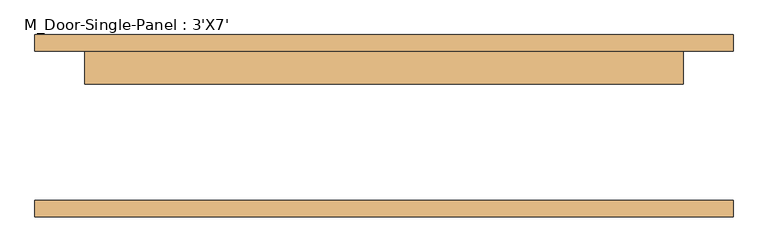
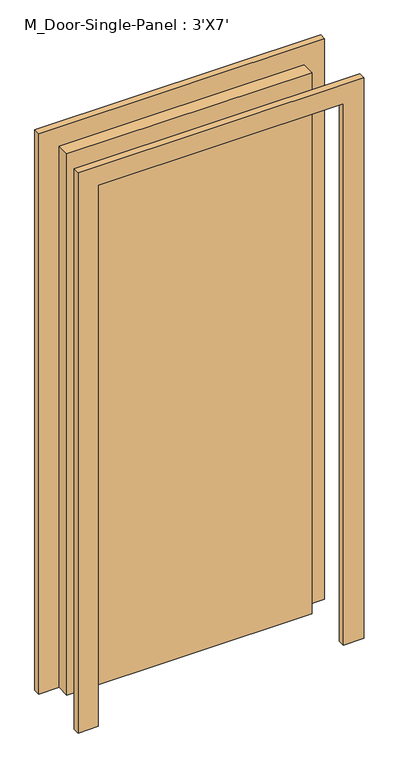
"""IFC4 building model written with IfcOpenShell, lengths in millimetres: door geometry, M_Door-Single-Panel : 3'X7'."""

from ifc_helpers import new_model, si_unit, frame, origin, origin_with_axes, place, context, project, spatial, polyline, outline, extrude, source, transform, mapped, element, save


def m_door_single_panel_3_x7_ed4aac83(model_context):
    return source(origin(), model_context, "Body", "SweptSolid", [
        extrude(outline(polyline([(457.2, 64.3), (-457.2, 64.3), (-457.2, 114.3), (457.2, 114.3), (457.2, 64.3)])), origin_with_axes(), (0.0, 0.0, 1.0), 2133.6),
        extrude(outline(polyline([(2209.8, 533.4), (2209.8, -533.4), (0.0, -533.4), (0.0, -457.2), (2133.6, -457.2), (2133.6, 457.2), (0.0, 457.2), (0.0, 533.4), (2209.8, 533.4)])), frame((0.0, -139.3, 0.0), z_axis=(0.0, 1.0, 0.0), x_axis=(0.0, 0.0, 1.0)), (0.0, 0.0, 1.0), 25.0),
        extrude(outline(polyline([(2209.8, -533.4), (0.0, -533.4), (0.0, -457.2), (2133.6, -457.2), (2133.6, 457.2), (0.0, 457.2), (0.0, 533.4), (2209.8, 533.4), (2209.8, -533.4)])), frame((0.0, 114.3, 0.0), z_axis=(0.0, 1.0, 0.0), x_axis=(0.0, 0.0, 1.0)), (0.0, 0.0, 1.0), 25.0),
    ])


if __name__ == "__main__":
    model = new_model("IFC4")
    model_context = context("Model", 3, world=origin())
    ifc_project = project(units=[si_unit("LENGTHUNIT", "METRE", prefix="MILLI")], contexts=[model_context])
    site = spatial("IfcSite", under=ifc_project)
    building = spatial("IfcBuilding", under=site)
    placement = place(None, origin())
    m_door_single_panel_3_x7_shape = m_door_single_panel_3_x7_ed4aac83(model_context)
    element("IfcDoor", 1, ObjectType="M_Door-Single-Panel : 3'X7'", at=placement, inside=building, context=model_context, shape_type="MappedRepresentation", body=[
        mapped(m_door_single_panel_3_x7_shape, transform((0.0, 0.0, 0.0), x_axis=(1.0, 0.0, 0.0), y_axis=(0.0, 1.0, 0.0), z_axis=(0.0, 0.0, 1.0))),
    ])
    save(model, "model.ifc")

# Revit data of these elements
# Type "M_Door-Single-Panel : 3'X7'"
#   Type Mark = "11"
#   Construction Type Id = "DOOR"
#   Assembly Code = "C1020300"
#   Analytic Construction = "Wooden"
#   Thickness = 0' - 1.9685"
#   Thermal Resistance (R) = 2.5876 (h·ft²·°F)/BTU
#   Swing Angle [instance default] = 90.00°
#   Heat Transfer Coefficient (U) = 0.3865 BTU/(h·ft²·°F)
#   Height = 7' - 0"
#   Trim Projection Ext = 0' - 0.98425"
#   Trim Projection Int = 0' - 0.98425"
#   Trim Width = 0' - 3.14961"
#   Width = 3' - 0"
#   Define Thermal Properties by = 1
#   Panel Material = Wood - Birch - Solid Stained Light Low Gloss
#   Trim Material = Paint - Sienna
#   Visual Light Transmittance = 0
#   Solar Heat Gain Coefficient = 0
#   Function = (empty or 0)
#   Wall Closure = (empty or 0)
# Element 1 (IfcDoor, "M_Door-Single-Panel : 3'X7'")
#   Materials on its faces: "Paint - Sienna", "Wood - Birch - Solid Stained Light Low Gloss"
# Materials
#   "Wood - Birch - Solid Stained Light Low Gloss": class "Wood", colour RGB 210 159 95, transparency 0, Cost = 0
#   "Paint - Sienna": colour RGB 118 70 51, transparency 0, Cost = 0
